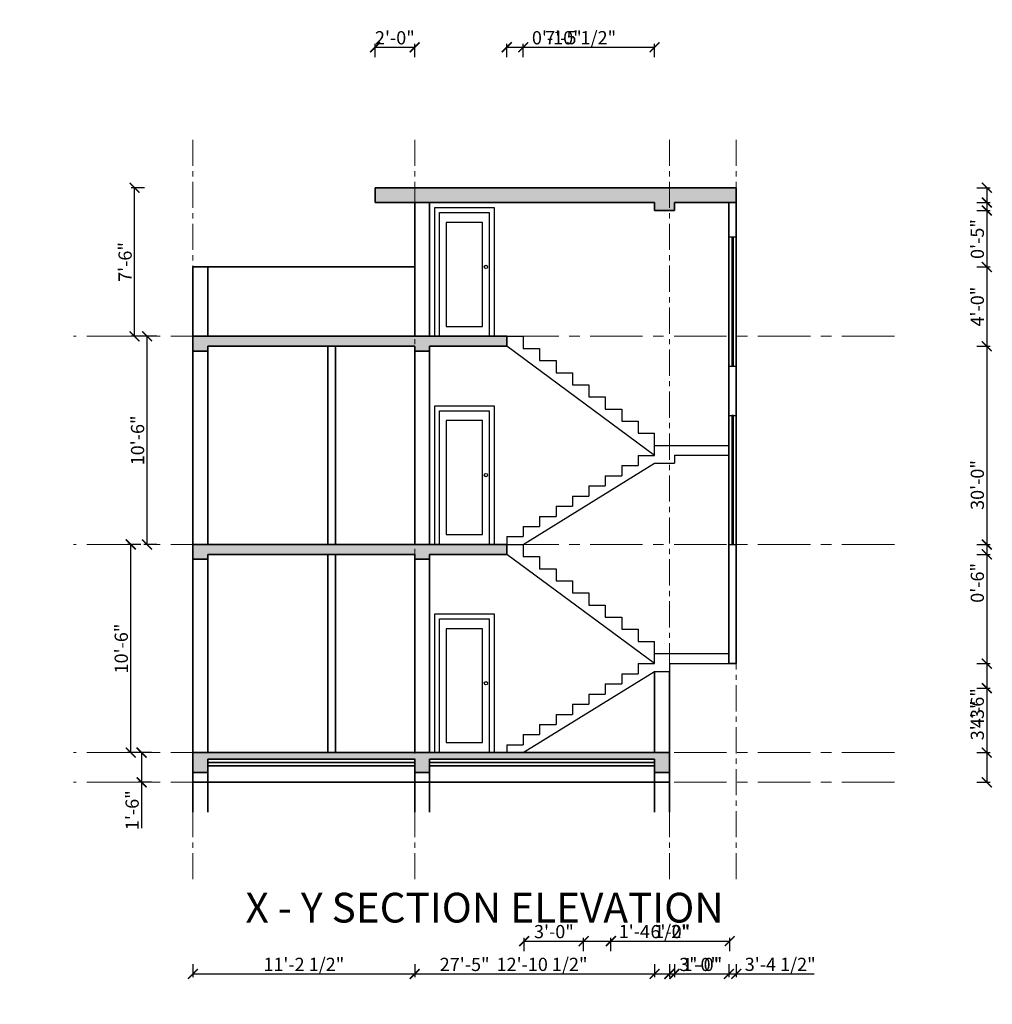
# Model space of a CAD drawing. Units: inches. Extents: x 378 to 1617, y 130 to 1256.
# Tile 5 of 5: x 1028 to 1617, y 660 to 1256. Entities that reach past the tile are written whole.
import ezdxf

# ---------------------------------------------------------------- set-up
doc = ezdxf.new("R2010")
doc.units = ezdxf.units.IN
doc.linetypes.add('CENTER', pattern=[50.8, 31.75, -6.35, 6.35, -6.35])
for name, color, linetype, lineweight in [('A-ANNO-TEXT', 7, 'Continuous', 25), ('A-ELEV-PATT', 8, 'Continuous', 13), ('A-SECT', 7, 'Continuous', 35), ('Dimensions', 153, 'Continuous', 18), ('Doors', 2, 'Continuous', 25), ('Grid lines', 7, 'CENTER', 18), ('Stairs', 40, 'Continuous', 25), ('Windows', 140, 'Continuous', 25)]:
    doc.layers.add(name, color=color, linetype=linetype, lineweight=lineweight)
doc.styles.get("Standard").update_dxf_attribs({"font": 'arial.ttf'})
doc.dimstyles.new('ISO-25', dxfattribs={"dimtxt": 8, "dimasz": 6, "dimexe": 2, "dimexo": 4, "dimtad": 1, "dimdec": 0, "dimlunit": 3, "dimtxsty": 'Standard', "dimblk": 'ARCHTICK', "dimcen": 2.5, "dimadec": 0, "dimazin": 0, "dimtfac": 1, "dimtdec": 0, "dimtmove": 0, "dimatfit": 3, "dimfxl": 6, "dimfxlon": 1, "dimarcsym": 0})

# ---------------------------------------------------------------- blocks, each defined once
blk = doc.blocks.new('*U17')
blk.add_lwpolyline([(3.12, 0.01), (0.12, 0.01), (0.12, 84.01), (36.12, 84.01), (36.12, 0.01), (33.12, 0.01)])
for points in [[(33.12, 80.99), (33.12, 0.01), (3.12, 0.01), (3.12, 80.99)], [(29.12, 6.01), (29.12, 74.99), (7.12, 74.99), (7.12, 6.01)]]:
    blk.add_lwpolyline(points, close=True)
blk.add_circle((31.12, 42.01), 1)
blk = doc.blocks.new('*U23')
blk.add_lwpolyline([(3.12, 0.01), (0.12, 0.01), (0.12, 78.01), (36.12, 78.01), (36.12, 0.01), (33.12, 0.01)])
for points in [[(33.12, 74.99), (33.12, 0.01), (3.12, 0.01), (3.12, 74.99)], [(29.12, 6.01), (29.12, 68.99), (7.12, 68.99), (7.12, 6.01)]]:
    blk.add_lwpolyline(points, close=True)
blk.add_circle((31.12, 42.01), 1)
blk = doc.blocks.new('_ArchTick')
at = {"color": 0, "linetype": 'ByBlock', "const_width": 0.15}
blk.add_lwpolyline([(-0.5, -0.5), (0.5, 0.5)], dxfattribs=at)
blk = doc.blocks.new('*D38')
at = {"layer": 'Defpoints', "color": 0, "transparency": 16777216}
for p in [(1128.48, 812.08), (1101.9, 794.08), (1128.48, 794.08)]:
    blk.add_point(p, dxfattribs=at)
at = {"layer": 'Dimensions', "color": 0, "lineweight": -2, "transparency": 16777216}
for p, q in [((1107.9, 812.08), (1099.9, 812.08)), ((1101.9, 812.08), (1101.9, 794.08)), ((1107.9, 794.08), (1099.9, 794.08)), ((1101.9, 794.08), (1101.9, 766.32))]:
    blk.add_line(p, q, dxfattribs=at)
at = {"layer": 'Dimensions', "color": 0, "lineweight": -2, "transparency": 16777216, "xscale": 6, "yscale": 6, "zscale": 6}
for p, rotation in [((1101.9, 812.08), 90), ((1101.9, 794.08), 270)]:
    blk.add_blockref('_ArchTick', p, dxfattribs=dict(at, rotation=rotation))
at = {"layer": 'Dimensions', "color": 0, "transparency": 16777216, "insert": (1097.19, 777.2), "char_height": 8, "attachment_point": 5, "rotation": 90}
blk.add_mtext('1\'-6"', dxfattribs=at)
blk = doc.blocks.new('*D36')
at = {"layer": 'Defpoints', "color": 0, "transparency": 16777216}
for p in [(1095.32, 938.08), (1128.48, 938.08), (1128.48, 812.08)]:
    blk.add_point(p, dxfattribs=at)
at = {"layer": 'Dimensions', "color": 0, "lineweight": -2, "transparency": 16777216}
for p, q in [((1101.32, 938.08), (1093.32, 938.08)), ((1095.32, 812.08), (1095.32, 938.08)), ((1101.32, 812.08), (1093.32, 812.08))]:
    blk.add_line(p, q, dxfattribs=at)
at = {"layer": 'Dimensions', "color": 0, "lineweight": -2, "transparency": 16777216, "xscale": 6, "yscale": 6, "zscale": 6}
for p, rotation in [((1095.32, 938.08), 90), ((1095.32, 812.08), 270)]:
    blk.add_blockref('_ArchTick', p, dxfattribs=dict(at, rotation=rotation))
at = {"layer": 'Dimensions', "color": 0, "transparency": 16777216, "insert": (1090.61, 875.08), "char_height": 8, "attachment_point": 5, "rotation": 90}
blk.add_mtext('10\'-6"', dxfattribs=at)
blk = doc.blocks.new('*D35')
at = {"layer": 'Defpoints', "color": 0, "transparency": 16777216}
for p in [(1105.19, 1064.08), (1128.48, 1064.08), (1128.48, 938.08)]:
    blk.add_point(p, dxfattribs=at)
at = {"layer": 'Dimensions', "color": 0, "lineweight": -2, "transparency": 16777216}
for p, q in [((1111.19, 1064.08), (1103.19, 1064.08)), ((1105.19, 938.08), (1105.19, 1064.08)), ((1111.19, 938.08), (1103.19, 938.08))]:
    blk.add_line(p, q, dxfattribs=at)
at = {"layer": 'Dimensions', "color": 0, "lineweight": -2, "transparency": 16777216, "xscale": 6, "yscale": 6, "zscale": 6}
for p, rotation in [((1105.19, 1064.08), 90), ((1105.19, 938.08), 270)]:
    blk.add_blockref('_ArchTick', p, dxfattribs=dict(at, rotation=rotation))
at = {"layer": 'Dimensions', "color": 0, "transparency": 16777216, "insert": (1100.48, 1001.08), "char_height": 8, "attachment_point": 5, "rotation": 90}
blk.add_mtext('10\'-6"', dxfattribs=at)
blk = doc.blocks.new('*D37')
at = {"layer": 'Defpoints', "color": 0, "transparency": 16777216}
for p in [(1097.63, 1154.08), (1128.48, 1154.08), (1128.48, 1064.08)]:
    blk.add_point(p, dxfattribs=at)
at = {"layer": 'Dimensions', "color": 0, "lineweight": -2, "transparency": 16777216}
for p, q in [((1103.63, 1154.08), (1095.63, 1154.08)), ((1097.63, 1064.08), (1097.63, 1154.08)), ((1103.63, 1064.08), (1095.63, 1064.08))]:
    blk.add_line(p, q, dxfattribs=at)
at = {"layer": 'Dimensions', "color": 0, "lineweight": -2, "transparency": 16777216, "xscale": 6, "yscale": 6, "zscale": 6}
for p, rotation in [((1097.63, 1154.08), 90), ((1097.63, 1064.08), 270)]:
    blk.add_blockref('_ArchTick', p, dxfattribs=dict(at, rotation=rotation))
at = {"layer": 'Dimensions', "color": 0, "transparency": 16777216, "insert": (1092.92, 1109.08), "char_height": 8, "attachment_point": 5, "rotation": 90}
blk.add_mtext('7\'-6"', dxfattribs=at)
blk = doc.blocks.new('*D71')
at = {"layer": 'Defpoints', "color": 0, "transparency": 16777216}
for p in [(1369.53, 697.95), (1333.53, 302.45), (1369.53, 302.45)]:
    blk.add_point(p, dxfattribs=at)
at = {"layer": 'Dimensions', "color": 0, "lineweight": -2, "transparency": 16777216}
for p, q in [((1333.53, 691.95), (1333.53, 699.95)), ((1333.53, 697.95), (1369.53, 697.95)), ((1369.53, 691.95), (1369.53, 699.95))]:
    blk.add_line(p, q, dxfattribs=at)
at = {"layer": 'Dimensions', "color": 0, "lineweight": -2, "transparency": 16777216, "xscale": 6, "yscale": 6, "zscale": 6, "rotation": 180}
blk.add_blockref('_ArchTick', (1333.53, 697.95), dxfattribs=at)
at = {"layer": 'Dimensions', "color": 0, "lineweight": -2, "transparency": 16777216, "xscale": 6, "yscale": 6, "zscale": 6}
blk.add_blockref('_ArchTick', (1369.53, 697.95), dxfattribs=at)
at = {"layer": 'Dimensions', "color": 0, "transparency": 16777216, "insert": (1351.53, 702.66), "char_height": 8, "attachment_point": 5}
blk.add_mtext('3\'-0"', dxfattribs=at)
blk = doc.blocks.new('*D72')
at = {"layer": 'Defpoints', "color": 0, "transparency": 16777216}
for p in [(1386.03, 697.95), (1369.53, 302.45), (1386.03, 302.45)]:
    blk.add_point(p, dxfattribs=at)
at = {"layer": 'Dimensions', "color": 0, "lineweight": -2, "transparency": 16777216}
for p, q in [((1369.53, 691.95), (1369.53, 699.95)), ((1369.53, 697.95), (1386.03, 697.95)), ((1386.03, 691.95), (1386.03, 699.95)), ((1386.03, 697.95), (1432.43, 697.95))]:
    blk.add_line(p, q, dxfattribs=at)
at = {"layer": 'Dimensions', "color": 0, "lineweight": -2, "transparency": 16777216, "xscale": 6, "yscale": 6, "zscale": 6, "rotation": 180}
blk.add_blockref('_ArchTick', (1369.53, 697.95), dxfattribs=at)
at = {"layer": 'Dimensions', "color": 0, "lineweight": -2, "transparency": 16777216, "xscale": 6, "yscale": 6, "zscale": 6}
blk.add_blockref('_ArchTick', (1386.03, 697.95), dxfattribs=at)
at = {"layer": 'Dimensions', "color": 0, "transparency": 16777216, "insert": (1412.23, 702.71), "char_height": 8, "attachment_point": 5}
blk.add_mtext('1\'-4 1/2"', dxfattribs=at)
blk = doc.blocks.new('*D73')
at = {"layer": 'Defpoints', "color": 0, "transparency": 16777216}
for p in [(1458.03, 697.95), (1386.03, 302.45), (1458.03, 302.45)]:
    blk.add_point(p, dxfattribs=at)
at = {"layer": 'Dimensions', "color": 0, "lineweight": -2, "transparency": 16777216}
for p, q in [((1386.03, 691.95), (1386.03, 699.95)), ((1386.03, 697.95), (1458.03, 697.95)), ((1458.03, 691.95), (1458.03, 699.95))]:
    blk.add_line(p, q, dxfattribs=at)
at = {"layer": 'Dimensions', "color": 0, "lineweight": -2, "transparency": 16777216, "xscale": 6, "yscale": 6, "zscale": 6, "rotation": 180}
blk.add_blockref('_ArchTick', (1386.03, 697.95), dxfattribs=at)
at = {"layer": 'Dimensions', "color": 0, "lineweight": -2, "transparency": 16777216, "xscale": 6, "yscale": 6, "zscale": 6}
blk.add_blockref('_ArchTick', (1458.03, 697.95), dxfattribs=at)
at = {"layer": 'Dimensions', "color": 0, "transparency": 16777216, "insert": (1422.03, 702.66), "char_height": 8, "attachment_point": 5}
blk.add_mtext('6\'-0"', dxfattribs=at)
blk = doc.blocks.new('*D76')
at = {"layer": 'Defpoints', "color": 0, "transparency": 16777216}
for p in [(883.53, 1106.08), (883.53, 1058.08), (1613.65, 1058.08)]:
    blk.add_point(p, dxfattribs=at)
at = {"layer": 'Dimensions', "color": 0, "lineweight": -2, "transparency": 16777216}
for p, q in [((1607.65, 1106.08), (1615.65, 1106.08)), ((1613.65, 1106.08), (1613.65, 1058.08)), ((1607.65, 1058.08), (1615.65, 1058.08))]:
    blk.add_line(p, q, dxfattribs=at)
at = {"layer": 'Dimensions', "color": 0, "lineweight": -2, "transparency": 16777216, "xscale": 6, "yscale": 6, "zscale": 6}
for p, rotation in [((1613.65, 1106.08), 90), ((1613.65, 1058.08), 270)]:
    blk.add_blockref('_ArchTick', p, dxfattribs=dict(at, rotation=rotation))
at = {"layer": 'Dimensions', "color": 0, "transparency": 16777216, "insert": (1608.94, 1082.08), "char_height": 8, "attachment_point": 5, "rotation": 90}
blk.add_mtext('4\'-0"', dxfattribs=at)
blk = doc.blocks.new('*D84')
at = {"layer": 'Defpoints', "color": 0, "transparency": 16777216}
for p in [(858.03, 851.08), (883.53, 812.08), (1613.65, 812.08)]:
    blk.add_point(p, dxfattribs=at)
at = {"layer": 'Dimensions', "color": 0, "lineweight": -2, "transparency": 16777216}
for p, q in [((1607.65, 851.08), (1615.65, 851.08)), ((1613.65, 851.08), (1613.65, 812.08)), ((1607.65, 812.08), (1615.65, 812.08))]:
    blk.add_line(p, q, dxfattribs=at)
at = {"layer": 'Dimensions', "color": 0, "lineweight": -2, "transparency": 16777216, "xscale": 6, "yscale": 6, "zscale": 6}
for p, rotation in [((1613.65, 851.08), 90), ((1613.65, 812.08), 270)]:
    blk.add_blockref('_ArchTick', p, dxfattribs=dict(at, rotation=rotation))
at = {"layer": 'Dimensions', "color": 0, "transparency": 16777216, "insert": (1608.94, 831.58), "char_height": 8, "attachment_point": 5, "rotation": 90}
blk.add_mtext('3\'-3"', dxfattribs=at)
blk = doc.blocks.new('*D87')
at = {"layer": 'Defpoints', "color": 0, "transparency": 16777216}
for p in [(1461.98, 1154.08), (1132.98, 794.08), (1461.98, 678.08)]:
    blk.add_point(p, dxfattribs=at)
at = {"layer": 'Dimensions', "color": 0, "lineweight": -2, "transparency": 16777216}
for p, q in [((1132.98, 684.08), (1132.98, 676.08)), ((1461.98, 684.08), (1461.98, 676.08)), ((1132.98, 678.08), (1461.98, 678.08))]:
    blk.add_line(p, q, dxfattribs=at)
at = {"layer": 'Dimensions', "color": 0, "lineweight": -2, "transparency": 16777216, "xscale": 6, "yscale": 6, "zscale": 6, "rotation": 180}
blk.add_blockref('_ArchTick', (1132.98, 678.08), dxfattribs=at)
at = {"layer": 'Dimensions', "color": 0, "lineweight": -2, "transparency": 16777216, "xscale": 6, "yscale": 6, "zscale": 6}
blk.add_blockref('_ArchTick', (1461.98, 678.08), dxfattribs=at)
at = {"layer": 'Dimensions', "color": 0, "transparency": 16777216, "insert": (1297.48, 682.79), "char_height": 8, "attachment_point": 5}
blk.add_mtext('27\'-5"', dxfattribs=at)
blk = doc.blocks.new('*D88')
at = {"layer": 'Defpoints', "color": 0, "transparency": 16777216}
for p in [(1461.98, 1154.08), (1421.48, 794.08), (1613.65, 794.08)]:
    blk.add_point(p, dxfattribs=at)
at = {"layer": 'Dimensions', "color": 0, "lineweight": -2, "transparency": 16777216}
for p, q in [((1607.65, 1154.08), (1615.65, 1154.08)), ((1613.65, 1154.08), (1613.65, 794.08)), ((1607.65, 794.08), (1615.65, 794.08))]:
    blk.add_line(p, q, dxfattribs=at)
at = {"layer": 'Dimensions', "color": 0, "lineweight": -2, "transparency": 16777216, "xscale": 6, "yscale": 6, "zscale": 6}
for p, rotation in [((1613.65, 1154.08), 90), ((1613.65, 794.08), 270)]:
    blk.add_blockref('_ArchTick', p, dxfattribs=dict(at, rotation=rotation))
at = {"layer": 'Dimensions', "color": 0, "transparency": 16777216, "insert": (1608.94, 974.08), "char_height": 8, "attachment_point": 5, "rotation": 90}
blk.add_mtext('30\'-0"', dxfattribs=at)
blk = doc.blocks.new('*D89')
at = {"layer": 'Defpoints', "color": 0, "transparency": 16777216}
for p in [(1267.23, 800.08), (1132.98, 794.08), (1267.23, 678.08)]:
    blk.add_point(p, dxfattribs=at)
at = {"layer": 'Dimensions', "color": 0, "lineweight": -2, "transparency": 16777216}
for p, q in [((1132.98, 684.08), (1132.98, 676.08)), ((1267.23, 684.08), (1267.23, 676.08)), ((1132.98, 678.08), (1267.23, 678.08))]:
    blk.add_line(p, q, dxfattribs=at)
at = {"layer": 'Dimensions', "color": 0, "lineweight": -2, "transparency": 16777216, "xscale": 6, "yscale": 6, "zscale": 6, "rotation": 180}
blk.add_blockref('_ArchTick', (1132.98, 678.08), dxfattribs=at)
at = {"layer": 'Dimensions', "color": 0, "lineweight": -2, "transparency": 16777216, "xscale": 6, "yscale": 6, "zscale": 6}
blk.add_blockref('_ArchTick', (1267.23, 678.08), dxfattribs=at)
at = {"layer": 'Dimensions', "color": 0, "transparency": 16777216, "insert": (1200.1, 682.84), "char_height": 8, "attachment_point": 5}
blk.add_mtext('11\'-2 1/2"', dxfattribs=at)
blk = doc.blocks.new('*D90')
at = {"layer": 'Defpoints', "color": 0, "transparency": 16777216}
for p in [(1267.23, 800.08), (1421.48, 794.08), (1421.48, 678.08)]:
    blk.add_point(p, dxfattribs=at)
at = {"layer": 'Dimensions', "color": 0, "lineweight": -2, "transparency": 16777216}
for p, q in [((1267.23, 684.08), (1267.23, 676.08)), ((1421.48, 684.08), (1421.48, 676.08)), ((1267.23, 678.08), (1421.48, 678.08))]:
    blk.add_line(p, q, dxfattribs=at)
at = {"layer": 'Dimensions', "color": 0, "lineweight": -2, "transparency": 16777216, "xscale": 6, "yscale": 6, "zscale": 6, "rotation": 180}
blk.add_blockref('_ArchTick', (1267.23, 678.08), dxfattribs=at)
at = {"layer": 'Dimensions', "color": 0, "lineweight": -2, "transparency": 16777216, "xscale": 6, "yscale": 6, "zscale": 6}
blk.add_blockref('_ArchTick', (1421.48, 678.08), dxfattribs=at)
at = {"layer": 'Dimensions', "color": 0, "transparency": 16777216, "insert": (1344.35, 682.84), "char_height": 8, "attachment_point": 5}
blk.add_mtext('12\'-10 1/2"', dxfattribs=at)
blk = doc.blocks.new('*D91')
at = {"layer": 'Defpoints', "color": 0, "transparency": 16777216}
for p in [(1461.98, 866.08), (1421.48, 794.08), (1461.98, 678.08)]:
    blk.add_point(p, dxfattribs=at)
at = {"layer": 'Dimensions', "color": 0, "lineweight": -2, "transparency": 16777216}
for p, q in [((1421.48, 684.08), (1421.48, 676.08)), ((1461.98, 684.08), (1461.98, 676.08)), ((1421.48, 678.08), (1461.98, 678.08)), ((1461.98, 678.08), (1509.13, 678.08))]:
    blk.add_line(p, q, dxfattribs=at)
at = {"layer": 'Dimensions', "color": 0, "lineweight": -2, "transparency": 16777216, "xscale": 6, "yscale": 6, "zscale": 6, "rotation": 180}
blk.add_blockref('_ArchTick', (1421.48, 678.08), dxfattribs=at)
at = {"layer": 'Dimensions', "color": 0, "lineweight": -2, "transparency": 16777216, "xscale": 6, "yscale": 6, "zscale": 6}
blk.add_blockref('_ArchTick', (1461.98, 678.08), dxfattribs=at)
at = {"layer": 'Dimensions', "color": 0, "transparency": 16777216, "insert": (1488.55, 682.85), "char_height": 8, "attachment_point": 5}
blk.add_mtext('3\'-4 1/2"', dxfattribs=at)
blk = doc.blocks.new('*D92')
at = {"layer": 'Defpoints', "color": 0, "transparency": 16777216}
for p in [(1267.23, 1239.08), (1243.23, 1154.08), (1267.23, 1145.08)]:
    blk.add_point(p, dxfattribs=at)
at = {"layer": 'Dimensions', "color": 0, "lineweight": -2, "transparency": 16777216}
for p, q in [((1243.23, 1233.08), (1243.23, 1241.08)), ((1267.23, 1233.08), (1267.23, 1241.08)), ((1243.23, 1239.08), (1267.23, 1239.08))]:
    blk.add_line(p, q, dxfattribs=at)
at = {"layer": 'Dimensions', "color": 0, "lineweight": -2, "transparency": 16777216, "xscale": 6, "yscale": 6, "zscale": 6, "rotation": 180}
blk.add_blockref('_ArchTick', (1243.23, 1239.08), dxfattribs=at)
at = {"layer": 'Dimensions', "color": 0, "lineweight": -2, "transparency": 16777216, "xscale": 6, "yscale": 6, "zscale": 6}
blk.add_blockref('_ArchTick', (1267.23, 1239.08), dxfattribs=at)
at = {"layer": 'Dimensions', "color": 0, "transparency": 16777216, "insert": (1255.23, 1243.79), "char_height": 8, "attachment_point": 5}
blk.add_mtext('2\'-0"', dxfattribs=at)
blk = doc.blocks.new('*D93')
at = {"layer": 'Defpoints', "color": 0, "transparency": 16777216}
for p in [(1243.23, 1154.08), (388.27, 1145.08), (1243.23, 1145.08)]:
    blk.add_point(p, dxfattribs=at)
at = {"layer": 'Dimensions', "color": 0, "lineweight": -2, "transparency": 16777216}
for p, q in [((394.27, 1154.08), (386.27, 1154.08)), ((388.27, 1154.08), (388.27, 1145.08)), ((394.27, 1145.08), (386.27, 1145.08)), ((388.27, 1145.08), (388.27, 1116.57))]:
    blk.add_line(p, q, dxfattribs=at)
at = {"layer": 'Dimensions', "color": 0, "lineweight": -2, "transparency": 16777216, "xscale": 6, "yscale": 6, "zscale": 6}
for p, rotation in [((388.27, 1154.08), 90), ((388.27, 1145.08), 270)]:
    blk.add_blockref('_ArchTick', p, dxfattribs=dict(at, rotation=rotation))
at = {"layer": 'Dimensions', "color": 0, "transparency": 16777216, "insert": (383.56, 1127.82), "char_height": 8, "attachment_point": 5, "rotation": 90}
blk.add_mtext('0\'-9"', dxfattribs=at)
blk = doc.blocks.new('*D94')
at = {"layer": 'Defpoints', "color": 0, "transparency": 16777216}
for p in [(1412.48, 1140.24), (1424.48, 1140.24), (1424.48, 678.08)]:
    blk.add_point(p, dxfattribs=at)
at = {"layer": 'Dimensions', "color": 0, "lineweight": -2, "transparency": 16777216}
for p, q in [((1412.48, 684.08), (1412.48, 676.08)), ((1424.48, 684.08), (1424.48, 676.08)), ((1412.48, 678.08), (1424.48, 678.08)), ((1424.48, 678.08), (1452.24, 678.08))]:
    blk.add_line(p, q, dxfattribs=at)
at = {"layer": 'Dimensions', "color": 0, "lineweight": -2, "transparency": 16777216, "xscale": 6, "yscale": 6, "zscale": 6, "rotation": 180}
blk.add_blockref('_ArchTick', (1412.48, 678.08), dxfattribs=at)
at = {"layer": 'Dimensions', "color": 0, "lineweight": -2, "transparency": 16777216, "xscale": 6, "yscale": 6, "zscale": 6}
blk.add_blockref('_ArchTick', (1424.48, 678.08), dxfattribs=at)
at = {"layer": 'Dimensions', "color": 0, "transparency": 16777216, "insert": (1441.36, 682.79), "char_height": 8, "attachment_point": 5}
blk.add_mtext('1\'-0"', dxfattribs=at)
blk = doc.blocks.new('*D95')
at = {"layer": 'Defpoints', "color": 0, "transparency": 16777216}
for p in [(1424.48, 1145.08), (1424.48, 1140.24), (1613.65, 1140.24)]:
    blk.add_point(p, dxfattribs=at)
at = {"layer": 'Dimensions', "color": 0, "lineweight": -2, "transparency": 16777216}
for p, q in [((1607.65, 1145.08), (1615.65, 1145.08)), ((1613.65, 1145.08), (1613.65, 1140.24)), ((1607.65, 1140.24), (1615.65, 1140.24)), ((1613.65, 1140.24), (1613.65, 1111.72))]:
    blk.add_line(p, q, dxfattribs=at)
at = {"layer": 'Dimensions', "color": 0, "lineweight": -2, "transparency": 16777216, "xscale": 6, "yscale": 6, "zscale": 6}
for p, rotation in [((1613.65, 1145.08), 90), ((1613.65, 1140.24), 270)]:
    blk.add_blockref('_ArchTick', p, dxfattribs=dict(at, rotation=rotation))
at = {"layer": 'Dimensions', "color": 0, "transparency": 16777216, "insert": (1608.94, 1122.98), "char_height": 8, "attachment_point": 5, "rotation": 90}
blk.add_mtext('0\'-5"', dxfattribs=at)
blk = doc.blocks.new('*D96')
at = {"layer": 'Defpoints', "color": 0, "transparency": 16777216}
for p in [(1322.98, 938.08), (1322.98, 932.08), (1613.65, 932.08)]:
    blk.add_point(p, dxfattribs=at)
at = {"layer": 'Dimensions', "color": 0, "lineweight": -2, "transparency": 16777216}
for p, q in [((1607.65, 938.08), (1615.65, 938.08)), ((1613.65, 938.08), (1613.65, 932.08)), ((1607.65, 932.08), (1615.65, 932.08)), ((1613.65, 932.08), (1613.65, 903.57))]:
    blk.add_line(p, q, dxfattribs=at)
at = {"layer": 'Dimensions', "color": 0, "lineweight": -2, "transparency": 16777216, "xscale": 6, "yscale": 6, "zscale": 6}
for p, rotation in [((1613.65, 938.08), 90), ((1613.65, 932.08), 270)]:
    blk.add_blockref('_ArchTick', p, dxfattribs=dict(at, rotation=rotation))
at = {"layer": 'Dimensions', "color": 0, "transparency": 16777216, "insert": (1608.94, 914.82), "char_height": 8, "attachment_point": 5, "rotation": 90}
blk.add_mtext('0\'-6"', dxfattribs=at)
blk = doc.blocks.new('*D97')
at = {"layer": 'Defpoints', "color": 0, "transparency": 16777216}
for p in [(1421.48, 866.08), (1457.48, 866.08), (1457.48, 678.08)]:
    blk.add_point(p, dxfattribs=at)
at = {"layer": 'Dimensions', "color": 0, "lineweight": -2, "transparency": 16777216}
for p, q in [((1421.48, 684.08), (1421.48, 676.08)), ((1457.48, 684.08), (1457.48, 676.08)), ((1421.48, 678.08), (1457.48, 678.08))]:
    blk.add_line(p, q, dxfattribs=at)
at = {"layer": 'Dimensions', "color": 0, "lineweight": -2, "transparency": 16777216, "xscale": 6, "yscale": 6, "zscale": 6, "rotation": 180}
blk.add_blockref('_ArchTick', (1421.48, 678.08), dxfattribs=at)
at = {"layer": 'Dimensions', "color": 0, "lineweight": -2, "transparency": 16777216, "xscale": 6, "yscale": 6, "zscale": 6}
blk.add_blockref('_ArchTick', (1457.48, 678.08), dxfattribs=at)
at = {"layer": 'Dimensions', "color": 0, "transparency": 16777216, "insert": (1439.48, 682.79), "char_height": 8, "attachment_point": 5}
blk.add_mtext('3\'-0"', dxfattribs=at)
blk = doc.blocks.new('*D98')
at = {"layer": 'Defpoints', "color": 0, "transparency": 16777216}
for p in [(1332.92, 1239.08), (1322.98, 816.8), (1332.92, 816.8)]:
    blk.add_point(p, dxfattribs=at)
at = {"layer": 'Dimensions', "color": 0, "lineweight": -2, "transparency": 16777216}
for p, q in [((1322.98, 1233.08), (1322.98, 1241.08)), ((1332.92, 1233.08), (1332.92, 1241.08)), ((1322.98, 1239.08), (1332.92, 1239.08)), ((1332.92, 1239.08), (1367.65, 1239.08))]:
    blk.add_line(p, q, dxfattribs=at)
at = {"layer": 'Dimensions', "color": 0, "lineweight": -2, "transparency": 16777216, "xscale": 6, "yscale": 6, "zscale": 6, "rotation": 180}
blk.add_blockref('_ArchTick', (1322.98, 1239.08), dxfattribs=at)
at = {"layer": 'Dimensions', "color": 0, "lineweight": -2, "transparency": 16777216, "xscale": 6, "yscale": 6, "zscale": 6}
blk.add_blockref('_ArchTick', (1332.92, 1239.08), dxfattribs=at)
at = {"layer": 'Dimensions', "color": 0, "transparency": 16777216, "insert": (1353.29, 1243.79), "char_height": 8, "attachment_point": 5}
blk.add_mtext('0\'-10"', dxfattribs=at)
blk = doc.blocks.new('*D99')
at = {"layer": 'Defpoints', "color": 0, "transparency": 16777216}
for p in [(1412.48, 865.94), (1322.98, 812.08), (1613.65, 812.08)]:
    blk.add_point(p, dxfattribs=at)
at = {"layer": 'Dimensions', "color": 0, "lineweight": -2, "transparency": 16777216}
for p, q in [((1607.65, 865.94), (1615.65, 865.94)), ((1613.65, 865.94), (1613.65, 812.08)), ((1607.65, 812.08), (1615.65, 812.08))]:
    blk.add_line(p, q, dxfattribs=at)
at = {"layer": 'Dimensions', "color": 0, "lineweight": -2, "transparency": 16777216, "xscale": 6, "yscale": 6, "zscale": 6}
for p, rotation in [((1613.65, 865.94), 90), ((1613.65, 812.08), 270)]:
    blk.add_blockref('_ArchTick', p, dxfattribs=dict(at, rotation=rotation))
at = {"layer": 'Dimensions', "color": 0, "transparency": 16777216, "insert": (1608.94, 839.01), "char_height": 8, "attachment_point": 5, "rotation": 90}
blk.add_mtext('4\'-6"', dxfattribs=at)
blk = doc.blocks.new('*D100')
at = {"layer": 'Defpoints', "color": 0, "transparency": 16777216}
for p in [(1412.48, 1239.08), (1322.98, 812.08), (1412.48, 812.08)]:
    blk.add_point(p, dxfattribs=at)
at = {"layer": 'Dimensions', "color": 0, "lineweight": -2, "transparency": 16777216}
for p, q in [((1322.98, 1233.08), (1322.98, 1241.08)), ((1412.48, 1233.08), (1412.48, 1241.08)), ((1322.98, 1239.08), (1412.48, 1239.08))]:
    blk.add_line(p, q, dxfattribs=at)
at = {"layer": 'Dimensions', "color": 0, "lineweight": -2, "transparency": 16777216, "xscale": 6, "yscale": 6, "zscale": 6, "rotation": 180}
blk.add_blockref('_ArchTick', (1322.98, 1239.08), dxfattribs=at)
at = {"layer": 'Dimensions', "color": 0, "lineweight": -2, "transparency": 16777216, "xscale": 6, "yscale": 6, "zscale": 6}
blk.add_blockref('_ArchTick', (1412.48, 1239.08), dxfattribs=at)
at = {"layer": 'Dimensions', "color": 0, "transparency": 16777216, "insert": (1367.73, 1243.84), "char_height": 8, "attachment_point": 5}
blk.add_mtext('7\'-5 1/2"', dxfattribs=at)

msp = doc.modelspace()

# ---------------------------------------------------------------- hatches: boundary and pattern name
at = {"layer": 'A-ELEV-PATT'}
h = msp.add_hatch(color=256, dxfattribs=at)
h.dxf.hatch_style = 1
h.paths.add_polyline_path([(1322.98, 1064.08), (1132.98, 1064.08), (1132.98, 1055.08), (1141.98, 1055.08), (1141.98, 1058.08), (1267.23, 1058.08), (1267.23, 1055.08), (1276.23, 1055.08), (1276.23, 1058.08), (1322.98, 1058.08)])
h.paths.add_polyline_path([(1322.98, 938.08), (1141.98, 938.08), (1132.98, 938.08), (1132.98, 929.08), (1141.98, 929.08), (1141.98, 932.08), (1267.23, 932.08), (1267.23, 929.08), (1276.23, 929.08), (1276.23, 932.08), (1322.98, 932.08)])
h.paths.add_polyline_path([(1461.98, 1154.08), (1243.23, 1154.08), (1243.23, 1145.08), (1412.48, 1145.08), (1412.48, 1140.24), (1424.48, 1140.24), (1424.48, 1145.08), (1461.98, 1145.08)])
h.paths.add_polyline_path([(1141.98, 808.08), (1267.23, 808.08), (1267.23, 800.08), (1276.23, 800.08), (1276.23, 808.08), (1412.48, 808.08), (1412.48, 800.08), (1421.48, 800.08), (1421.48, 812.08), (1412.48, 812.08), (1141.98, 812.08), (1132.98, 812.08), (1132.98, 800.08), (1141.98, 800.08)])
h = msp.add_hatch(dxfattribs=at)
h.set_pattern_fill('GOST_GLASS', color=256, scale=0.8)
h.paths.add_polyline_path([(565.53, 1003.08), (555.03, 1003.08), (555.03, 951.08), (565.53, 951.08)])
h.paths.add_polyline_path([(577.03, 1003.08), (566.53, 1003.08), (566.53, 951.08), (577.03, 951.08)])
h.paths.add_polyline_path([(566.53, 1015.07), (566.53, 1004.08), (577.03, 1004.08, 0.400957)])
h.paths.add_polyline_path([(565.53, 1015.07, 0.400957), (555.03, 1004.08), (565.53, 1004.08)])
h.paths.add_polyline_path([(565.53, 950.08), (555.03, 950.08, 0.400957), (565.53, 939.09)])
h.paths.add_polyline_path([(577.03, 950.08), (566.53, 950.08), (566.53, 939.09, 0.400957)])
h.paths.add_polyline_path([(577.03, 1111.08), (566.53, 1111.08), (566.53, 1059.08), (577.03, 1059.08)])
h.paths.add_polyline_path([(565.53, 1111.08), (555.03, 1111.08), (555.03, 1059.08), (565.53, 1059.08)])
h.paths.add_polyline_path([(565.53, 1058.08), (555.03, 1058.08, 0.400957), (565.53, 1047.09)])
h.paths.add_polyline_path([(577.03, 1058.08), (566.53, 1058.08), (566.53, 1047.09, 0.400957)])
h.paths.add_polyline_path([(566.53, 1123.07), (566.53, 1112.08), (577.03, 1112.08, 0.400957)])
h.paths.add_polyline_path([(565.53, 1123.07, 0.400957), (555.03, 1112.08), (565.53, 1112.08)])
h.paths.add_polyline_path([(683.53, 1013.08), (670.03, 1013.08), (656.53, 1013.08), (656.53, 979.08), (683.53, 979.08)])
h.paths.add_polyline_path([(654.53, 1013.08), (642.03, 1013.08), (642.03, 979.08), (654.53, 979.08)])
h.paths.add_polyline_path([(669.03, 1023.08), (642.03, 1023.08), (642.03, 1015.08), (669.03, 1015.08)])
h.paths.add_polyline_path([(698.03, 1013.08), (685.53, 1013.08), (685.53, 979.08), (698.03, 979.08)])
h.paths.add_polyline_path([(698.03, 1023.08), (671.03, 1023.08), (671.03, 1015.08), (698.03, 1015.08)])
h.paths.add_polyline_path([(804.03, 1013.08), (788.03, 1013.08), (788.03, 979.08), (804.03, 979.08)])
h.paths.add_polyline_path([(821.03, 1013.08), (805.03, 1013.08), (805.03, 979.08), (821.03, 979.08)])
h.paths.add_polyline_path([(821.03, 1023.08), (788.03, 1023.08), (788.03, 1015.08), (821.03, 1015.08)])
h.paths.add_polyline_path([(839.03, 1013.08), (823.03, 1013.08), (823.03, 979.08), (839.03, 979.08)])
h.paths.add_polyline_path([(856.03, 1013.08), (840.03, 1013.08), (840.03, 979.08), (856.03, 979.08)])
h.paths.add_polyline_path([(856.03, 1023.08), (823.03, 1023.08), (823.03, 1015.08), (856.03, 1015.08)])
h.paths.add_polyline_path([(683.53, 887.08), (670.03, 887.08), (656.53, 887.08), (656.53, 853.08), (683.53, 853.08)])
h.paths.add_polyline_path([(654.53, 887.08), (642.03, 887.08), (642.03, 853.08), (654.53, 853.08)])
h.paths.add_polyline_path([(698.03, 887.08), (685.53, 887.08), (685.53, 853.08), (698.03, 853.08)])
h.paths.add_polyline_path([(698.03, 897.08), (671.03, 897.08), (671.03, 889.08), (698.03, 889.08)])
h.paths.add_polyline_path([(669.03, 897.08), (642.03, 897.08), (642.03, 889.08), (669.03, 889.08)])
h.paths.add_polyline_path([(804.03, 887.08), (788.03, 887.08), (788.03, 853.08), (804.03, 853.08)])
h.paths.add_polyline_path([(821.03, 887.08), (805.03, 887.08), (805.03, 853.08), (821.03, 853.08)])
h.paths.add_polyline_path([(839.03, 887.08), (823.03, 887.08), (823.03, 853.08), (839.03, 853.08)])
h.paths.add_polyline_path([(856.03, 887.08), (840.03, 887.08), (840.03, 853.08), (856.03, 853.08)])
h.paths.add_polyline_path([(856.03, 897.08), (823.03, 897.08), (823.03, 889.08), (856.03, 889.08)])
h.paths.add_polyline_path([(821.03, 897.08), (788.03, 897.08), (788.03, 889.08), (821.03, 889.08)])
h.paths.add_polyline_path([(1460.23, 1016.08), (1459.23, 1016.08), (1459.23, 938.08), (1460.23, 938.08)])
h.paths.add_polyline_path([(1460.23, 1124.08), (1459.23, 1124.08), (1459.23, 1046.08), (1460.23, 1046.08)])

# ---------------------------------------------------------------- linework, layer by layer
at = {"layer": 'A-SECT'}
for p, q in [((1461.98, 1154.08), (1243.23, 1154.08)), ((1243.23, 1145.08), (1243.23, 1154.08)), ((1461.98, 866.08), (1461.98, 1154.08)), ((1412.48, 1145.08), (1243.23, 1145.08)), ((1267.23, 1064.08), (1267.23, 1145.08)), ((1276.23, 1064.08), (1276.23, 1145.08)), ((1412.48, 1145.08), (1412.48, 1140.24)), ((1461.98, 1145.08), (1424.48, 1145.08)), ((1424.48, 1140.24), (1424.48, 1145.08)), ((1457.48, 866.08), (1457.48, 1145.08)), ((1412.48, 1140.24), (1424.48, 1140.24)), ((1132.98, 776.08), (1132.98, 1106.08)), ((1132.98, 1106.08), (1267.23, 1106.08)), ((1141.98, 1064.08), (1141.98, 1106.08)), ((1132.98, 1064.08), (1322.98, 1064.08)), ((1322.98, 1058.08), (1322.98, 1064.08)), ((1132.98, 1055.08), (1141.98, 1055.08)), ((1141.98, 1058.08), (1267.23, 1058.08)), ((1141.98, 938.08), (1141.98, 1058.08)), ((1214.73, 938.08), (1214.73, 1058.08)), ((1219.23, 938.08), (1219.23, 1058.08)), ((1267.23, 938.08), (1267.23, 1058.08)), ((1267.23, 1055.08), (1276.23, 1055.08)), ((1276.23, 938.08), (1276.23, 1058.08)), ((1276.23, 1058.08), (1322.98, 1058.08)), ((1141.98, 938.08), (1132.98, 938.08)), ((1141.98, 938.08), (1322.98, 938.08)), ((1276.23, 938.08), (1267.23, 938.08)), ((1322.98, 932.08), (1322.98, 938.08)), ((1141.98, 932.08), (1267.23, 932.08)), ((1141.98, 812.08), (1141.98, 932.08)), ((1214.73, 812.08), (1214.73, 932.08)), ((1219.23, 812.08), (1219.23, 932.08)), ((1267.23, 812.08), (1267.23, 932.08)), ((1276.23, 812.08), (1276.23, 932.08)), ((1276.23, 932.08), (1322.98, 932.08)), ((1132.98, 929.08), (1141.98, 929.08)), ((1267.23, 929.08), (1276.23, 929.08)), ((1457.48, 866.08), (1461.98, 866.08)), ((1412.48, 812.08), (1412.48, 861.24)), ((1421.48, 776.08), (1421.48, 861.24)), ((1141.98, 812.08), (1132.98, 812.08)), ((1141.98, 812.08), (1412.48, 812.08)), ((1421.48, 812.08), (1412.48, 812.08)), ((1421.48, 800.08), (1421.48, 812.08)), ((1141.98, 776.08), (1141.98, 808.08)), ((1141.98, 808.08), (1267.23, 808.08)), ((1141.98, 800.08), (1141.98, 808.08)), ((1141.98, 806.08), (1267.23, 806.08)), ((1267.23, 776.08), (1267.23, 808.08)), ((1276.23, 776.08), (1276.23, 808.08)), ((1276.23, 808.08), (1412.48, 808.08)), ((1276.23, 806.08), (1412.48, 806.08)), ((1412.48, 776.08), (1412.48, 808.08)), ((1132.98, 800.08), (1141.98, 800.08)), ((1141.98, 804.08), (1267.23, 804.08)), ((1267.23, 800.08), (1276.23, 800.08)), ((1276.23, 804.08), (1412.48, 804.08)), ((1412.48, 800.08), (1421.48, 800.08)), ((1132.98, 794.08), (1421.48, 794.08))]:
    msp.add_line(p, q, dxfattribs=at)
at = {"layer": 'Grid lines', "ltscale": 0.5}
for p, q in [((1132.98, 1183.08), (1132.98, 734.08)), ((1267.23, 1183.08), (1267.23, 734.08)), ((1421.48, 1183.08), (1421.48, 734.08)), ((1461.98, 1183.08), (1461.98, 734.08))]:
    msp.add_line(p, q, dxfattribs=at)
at = {"layer": 'Grid lines'}
for p, q in [((1557.65, 1064.08), (1060.71, 1064.08)), ((1557.65, 938.08), (1060.71, 938.08)), ((1557.65, 812.08), (1060.71, 812.08)), ((1557.65, 794.08), (1060.71, 794.08))]:
    msp.add_line(p, q, dxfattribs=at)
at = {"layer": 'Stairs'}
for p, q in [((1322.98, 1064.08), (1332.92, 1064.08)), ((1332.92, 1064.08), (1332.92, 1056.75)), ((1412.48, 991.94), (1322.98, 1058.08)), ((1332.92, 1056.75), (1342.87, 1056.75)), ((1342.87, 1056.75), (1342.87, 1049.41)), ((1342.87, 1049.41), (1352.81, 1049.41)), ((1352.81, 1049.41), (1352.81, 1042.08)), ((1352.81, 1042.08), (1362.76, 1042.08)), ((1362.76, 1042.08), (1362.76, 1034.75)), ((1362.76, 1034.75), (1372.7, 1034.75)), ((1372.7, 1034.75), (1372.7, 1027.41)), ((1372.7, 1027.41), (1382.64, 1027.41)), ((1382.64, 1027.41), (1382.64, 1020.08)), ((1382.64, 1020.08), (1392.59, 1020.08)), ((1392.59, 1020.08), (1392.59, 1012.75)), ((1392.59, 1012.75), (1402.53, 1012.75)), ((1402.53, 1012.75), (1402.53, 1005.41)), ((1402.53, 1005.41), (1412.48, 1005.41)), ((1412.48, 991.94), (1412.48, 1005.41)), ((1412.48, 998.08), (1457.48, 998.08)), ((1402.53, 991.94), (1412.48, 991.94)), ((1402.53, 991.94), (1402.53, 985.8)), ((1424.48, 992.08), (1457.48, 992.08)), ((1424.48, 992.08), (1424.48, 987.24)), ((1332.89, 938.08), (1412.48, 987.24)), ((1392.59, 985.8), (1402.53, 985.8)), ((1392.59, 985.8), (1392.59, 979.66)), ((1412.48, 987.24), (1424.48, 987.24)), ((1382.64, 979.66), (1392.59, 979.66)), ((1382.64, 979.66), (1382.64, 973.51)), ((1372.7, 973.51), (1382.64, 973.51)), ((1372.7, 973.51), (1372.7, 967.37)), ((1362.76, 967.37), (1372.7, 967.37)), ((1362.76, 967.37), (1362.76, 961.23)), ((1352.81, 961.23), (1362.76, 961.23)), ((1352.81, 961.23), (1352.81, 955.09)), ((1342.87, 955.09), (1352.81, 955.09)), ((1342.87, 955.09), (1342.87, 948.95)), ((1332.92, 948.95), (1342.87, 948.95)), ((1332.92, 948.95), (1332.92, 942.8)), ((1322.98, 942.8), (1332.92, 942.8)), ((1322.98, 942.8), (1322.98, 938.08)), ((1322.98, 938.08), (1332.92, 938.08)), ((1332.92, 938.08), (1332.92, 930.75)), ((1412.48, 865.94), (1322.98, 932.08)), ((1332.92, 930.75), (1342.87, 930.75)), ((1342.87, 930.75), (1342.87, 923.41)), ((1342.87, 923.41), (1352.81, 923.41)), ((1352.81, 923.41), (1352.81, 916.08)), ((1352.81, 916.08), (1362.76, 916.08)), ((1362.76, 916.08), (1362.76, 908.75)), ((1362.76, 908.75), (1372.7, 908.75)), ((1372.7, 908.75), (1372.7, 901.41)), ((1372.7, 901.41), (1382.64, 901.41)), ((1382.64, 901.41), (1382.64, 894.08)), ((1382.64, 894.08), (1392.59, 894.08)), ((1392.59, 894.08), (1392.59, 886.75)), ((1392.59, 886.75), (1402.53, 886.75)), ((1402.53, 886.75), (1402.53, 879.41)), ((1402.53, 879.41), (1412.48, 879.41)), ((1412.48, 865.94), (1412.48, 879.41)), ((1412.48, 872.08), (1457.48, 872.08)), ((1402.53, 865.94), (1412.48, 865.94)), ((1402.53, 865.94), (1402.53, 859.8)), ((1421.48, 866.08), (1457.48, 866.08)), ((1421.48, 866.08), (1421.48, 861.24)), ((1332.89, 812.08), (1412.48, 861.24)), ((1392.59, 859.8), (1402.53, 859.8)), ((1392.59, 859.8), (1392.59, 853.66)), ((1412.48, 861.24), (1421.48, 861.24)), ((1382.64, 853.66), (1392.59, 853.66)), ((1382.64, 853.66), (1382.64, 847.51)), ((1372.7, 847.51), (1382.64, 847.51)), ((1372.7, 847.51), (1372.7, 841.37)), ((1362.76, 841.37), (1372.7, 841.37)), ((1362.76, 841.37), (1362.76, 835.23)), ((1352.81, 835.23), (1362.76, 835.23)), ((1352.81, 835.23), (1352.81, 829.09)), ((1342.87, 829.09), (1352.81, 829.09)), ((1342.87, 829.09), (1342.87, 822.95)), ((1332.92, 822.95), (1342.87, 822.95)), ((1332.92, 822.95), (1332.92, 816.8)), ((1322.98, 816.8), (1332.92, 816.8)), ((1322.98, 816.8), (1322.98, 812.08))]:
    msp.add_line(p, q, dxfattribs=at)
at = {"layer": 'Windows'}
for p, q in [((1461.98, 1124.08), (1457.48, 1124.08)), ((1457.48, 1046.08), (1461.98, 1046.08)), ((1457.48, 1016.08), (1461.98, 1016.08)), ((1457.48, 938.08), (1461.98, 938.08))]:
    msp.add_line(p, q, dxfattribs=at)
for points in [[(1459.23, 1046.08), (1460.23, 1046.08), (1460.23, 1124.08), (1459.23, 1124.08)], [(1459.23, 938.08), (1460.23, 938.08), (1460.23, 1016.08), (1459.23, 1016.08)]]:
    msp.add_lwpolyline(points, close=True, dxfattribs=at)

# ---------------------------------------------------------------- block references
at = {"layer": 'Doors'}
for name, p in [('*U23', (1279.23, 1064.08)), ('*U17', (1279.23, 938.08)), ('*U17', (1279.23, 812.08))]:
    msp.add_blockref(name, p, dxfattribs=at)

# ---------------------------------------------------------------- texts
at = {"layer": 'A-ANNO-TEXT', "insert": (1136.57, 727.2), "char_height": 18, "attachment_point": 1}
msp.add_mtext_dynamic_manual_height_columns('\\pxqc;{\\fTimes New Roman|b0|i0|c0|p18;X - Y SECTION ELEVATION}', width=345.962, gutter_width=12.5, heights=[0], dxfattribs=at)

# ---------------------------------------------------------------- dimensions: what is measured, and where the dimension line sits
at = {"layer": 'Dimensions'}
for base, p1, p2, picture, middle in [((1412.48, 1239.08), (1322.98, 812.08), (1412.48, 812.08), '*D100', (1367.73, 1243.84)), ((1267.23, 1239.08), (1243.23, 1154.08), (1267.23, 1145.08), '*D92', (1255.23, 1243.79)), ((1332.92, 1239.08), (1322.98, 816.8), (1332.92, 816.8), '*D98', (1353.29, 1243.79)), ((1461.98, 678.08), (1132.98, 794.08), (1461.98, 1154.08), '*D87', (1297.48, 682.79)), ((1424.48, 678.08), (1412.48, 1140.24), (1424.48, 1140.24), '*D94', (1441.36, 682.79)), ((1461.98, 678.08), (1421.48, 794.08), (1461.98, 866.08), '*D91', (1488.55, 682.85)), ((1457.48, 678.08), (1421.48, 866.08), (1457.48, 866.08), '*D97', (1439.48, 682.79)), ((1267.227651, 678.081639), (1132.977651, 794.081639), (1267.227651, 800.081639), '*D89', (1200.102651, 682.84306465)), ((1421.477651, 678.081639), (1267.227651, 800.081639), (1421.477651, 794.081639), '*D90', (1344.352651, 682.84306465)), ((1386.03, 697.95), (1369.53, 302.45), (1386.03, 302.45), '*D72', (1412.23, 702.71)), ((1369.53, 697.95), (1333.53, 302.45), (1369.53, 302.45), '*D71', (1351.53, 702.66)), ((1458.03, 697.95), (1386.03, 302.45), (1458.03, 302.45), '*D73', (1422.03, 702.66))]:
    dim = msp.add_linear_dim(base=base, p1=p1, p2=p2, dimstyle='ISO-25', override={"dimdec": 1, "dimlfac": 1, "dimrnd": 0, "dimzin": 1, "dimdsep": 46, "dimlunit": 4, "dimfrac": 2}, dxfattribs=at)
    dim.commit()
    dim.dimension.update_dxf_attribs({"geometry": picture, "text_midpoint": middle})
for base, p1, p2, override, picture, middle in [((388.27, 1145.08), (1243.23, 1154.08), (1243.23, 1145.08), {"dimdec": 1, "dimlfac": 1, "dimrnd": 0, "dimzin": 1, "dimdsep": 46, "dimlunit": 4, "dimfrac": 2}, '*D93', (383.56, 1127.82)), ((1097.63, 1154.08), (1128.48, 1064.08), (1128.48, 1154.08), {"dimclrd": 0, "dimclre": 0, "dimclrt": 0}, '*D37', (1092.92, 1109.08)), ((1613.65, 794.08), (1461.98, 1154.08), (1421.48, 794.08), {"dimdec": 1, "dimlfac": 1, "dimrnd": 0, "dimzin": 1, "dimdsep": 46, "dimlunit": 4, "dimfrac": 2}, '*D88', (1608.94, 974.08)), ((1613.65, 1140.24), (1424.48, 1145.08), (1424.48, 1140.24), {"dimdec": 1, "dimlfac": 1, "dimrnd": 0, "dimzin": 1, "dimdsep": 46, "dimlunit": 4, "dimfrac": 2}, '*D95', (1608.94, 1122.98)), ((1613.65, 1058.08), (883.53, 1106.08), (883.53, 1058.08), {"dimdec": 1, "dimlfac": 1, "dimrnd": 0, "dimzin": 1, "dimdsep": 46, "dimlunit": 4, "dimfrac": 2}, '*D76', (1608.94, 1082.08)), ((1105.19, 1064.08), (1128.48, 938.08), (1128.48, 1064.08), {"dimclrd": 0, "dimclre": 0, "dimclrt": 0}, '*D35', (1100.48, 1001.08)), ((1095.32, 938.08), (1128.48, 812.08), (1128.48, 938.08), {"dimclrd": 0, "dimclre": 0, "dimclrt": 0}, '*D36', (1090.61, 875.08)), ((1613.65, 932.08), (1322.98, 938.08), (1322.98, 932.08), {"dimdec": 1, "dimlfac": 1, "dimrnd": 0, "dimzin": 1, "dimdsep": 46, "dimlunit": 4, "dimfrac": 2}, '*D96', (1608.94, 914.82)), ((1613.65, 812.08), (1412.48, 865.94), (1322.98, 812.08), {"dimdec": 1, "dimlfac": 1, "dimrnd": 0, "dimzin": 1, "dimdsep": 46, "dimlunit": 4, "dimfrac": 2}, '*D99', (1608.94, 839.01)), ((1613.65, 812.08), (858.03, 851.08), (883.53, 812.08), {"dimdec": 1, "dimlfac": 1, "dimrnd": 0, "dimzin": 1, "dimdsep": 46, "dimlunit": 4, "dimfrac": 2}, '*D84', (1608.94, 831.58)), ((1101.9, 794.08), (1128.48, 812.08), (1128.48, 794.08), {"dimclrd": 0, "dimclre": 0, "dimclrt": 0}, '*D38', (1097.19, 777.2))]:
    dim = msp.add_linear_dim(base=base, p1=p1, p2=p2, angle=90, dimstyle='ISO-25', override=override, dxfattribs=at)
    dim.commit()
    dim.dimension.update_dxf_attribs({"geometry": picture, "text_midpoint": middle})

doc.saveas('drawing.dxf')
